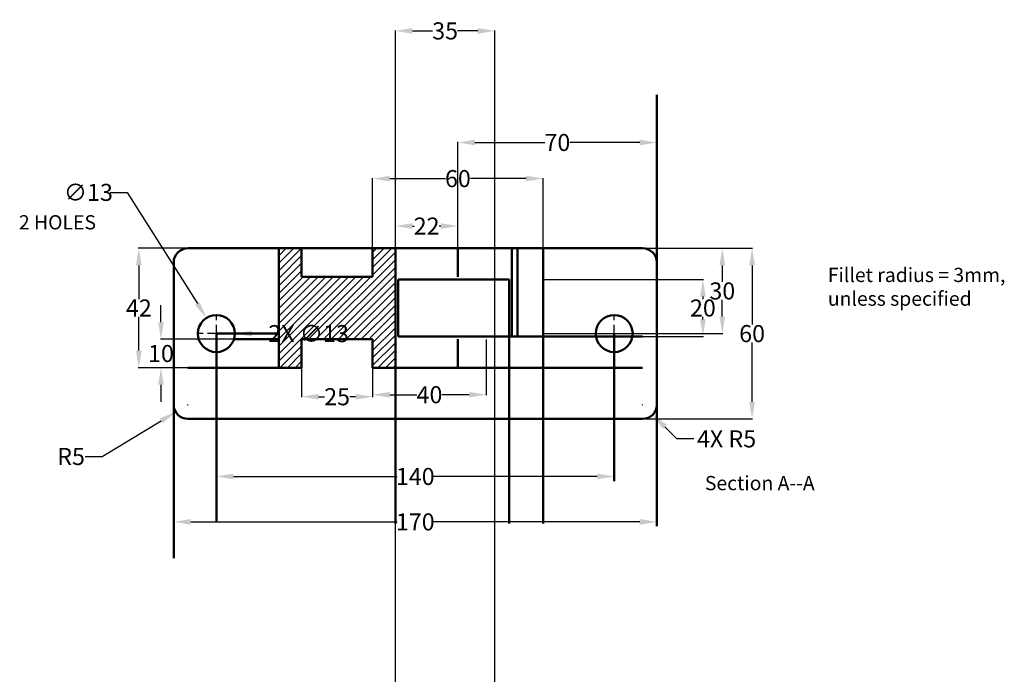
# Model space of a CAD drawing. Units: inches. Extents: x 537 to 975, y 162 to 623.
# Tile 2 of 2: x 537 to 883, y 393 to 623. Entities that reach past the tile are written whole.
import ezdxf

# ---------------------------------------------------------------- set-up
doc = ezdxf.new("R2010")
doc.units = ezdxf.units.IN
doc.header["$LTSCALE"] = 5
doc.header["$MEASUREMENT"] = 0
doc.linetypes.add('HIDDEN2', pattern=[0.1875, 0.125, -0.0625])
for name, color, linetype, lineweight in [('M-DIMS', 2, 'Continuous', 25), ('M-HATC', 8, 'Continuous', 18), ('M-HIDN', 4, 'HIDDEN2', 25), ('M-OUTL', 7, 'Continuous', 50), ('M-TEXT', 3, 'Continuous', 25)]:
    doc.layers.add(name, color=color, linetype=linetype, lineweight=lineweight)
doc.styles.get("Standard").update_dxf_attribs({"font": 'arial.ttf'})
doc.dimstyles.get("Standard").update_dxf_attribs({"dimtxt": 6, "dimasz": 6, "dimexe": 0.18, "dimexo": 0.0625, "dimgap": 0.09, "dimtad": 0, "dimtih": 1, "dimtoh": 1, "dimdec": 0, "dimzin": 0, "dimdsep": 46, "dimtxsty": 'Standard', "dimcen": 0.09, "dimadec": 0, "dimazin": 0, "dimtfac": 1, "dimtdec": 0, "dimtofl": 0, "dimtmove": 0, "dimatfit": 3, "dimfxl": 1, "dimtolj": 1, "dimtzin": 0, "dimarcsym": 0})

# ---------------------------------------------------------------- blocks, each defined once
blk = doc.blocks.new('*D1')
at = {"layer": 'Defpoints', "color": 0, "lineweight": 30, "transparency": 16777216}
for p in [(605.92, 483.04), (745.92, 483.83), (745.92, 462.8)]:
    blk.add_point(p, dxfattribs=at)
at = {"layer": 'M-DIMS', "color": 0, "lineweight": -2, "transparency": 16777216}
for p, q in [((605.92, 482.98), (605.92, 462.62)), ((745.92, 483.77), (745.92, 462.62)), ((611.92, 462.8), (669.49, 462.8)), ((739.92, 462.8), (682.34, 462.8))]:
    blk.add_line(p, q, dxfattribs=at)
at = {"layer": 'M-DIMS', "color": 0, "lineweight": 30, "transparency": 16777216}
for points in [[(611.92, 463.8), (611.92, 461.8), (605.92, 462.8)], [(739.92, 463.8), (739.92, 461.8), (745.92, 462.8)]]:
    blk.add_solid(points, dxfattribs=at)
at = {"layer": 'M-DIMS', "color": 0, "transparency": 16777216, "insert": (675.92, 462.8), "char_height": 6, "attachment_point": 5}
blk.add_mtext('\\A1;140', dxfattribs=at)
blk = doc.blocks.new('*D2')
at = {"layer": 'Defpoints', "color": 0, "lineweight": 30, "transparency": 16777216}
for p in [(760.92, 451.49), (590.92, 448.29), (760.92, 446.82)]:
    blk.add_point(p, dxfattribs=at)
at = {"layer": 'M-DIMS', "color": 0, "lineweight": -2, "transparency": 16777216}
for p, q in [((760.92, 451.43), (760.92, 446.64)), ((590.92, 448.23), (590.92, 446.64)), ((596.92, 446.82), (669.49, 446.82)), ((754.92, 446.82), (682.34, 446.82))]:
    blk.add_line(p, q, dxfattribs=at)
at = {"layer": 'M-DIMS', "color": 0, "lineweight": 30, "transparency": 16777216}
for points in [[(596.92, 447.82), (596.92, 445.82), (590.92, 446.82)], [(754.92, 447.82), (754.92, 445.82), (760.92, 446.82)]]:
    blk.add_solid(points, dxfattribs=at)
at = {"layer": 'M-DIMS', "color": 0, "transparency": 16777216, "insert": (675.92, 446.82), "char_height": 6, "attachment_point": 5}
blk.add_mtext('\\A1;170', dxfattribs=at)
blk = doc.blocks.new('*D3')
at = {"layer": 'Defpoints', "color": 0, "lineweight": 30, "transparency": 16777216}
for p in [(660.92, 511.04), (700.92, 511.04), (700.92, 491.55)]:
    blk.add_point(p, dxfattribs=at)
at = {"layer": 'M-DIMS', "color": 0, "lineweight": -2, "transparency": 16777216}
for p, q in [((660.92, 510.98), (660.92, 491.37)), ((700.92, 510.98), (700.92, 491.37)), ((666.92, 491.55), (676.42, 491.55)), ((694.92, 491.55), (685.41, 491.55))]:
    blk.add_line(p, q, dxfattribs=at)
at = {"layer": 'M-DIMS', "color": 0, "lineweight": 30, "transparency": 16777216}
for points in [[(666.92, 492.55), (666.92, 490.55), (660.92, 491.55)], [(694.92, 492.55), (694.92, 490.55), (700.92, 491.55)]]:
    blk.add_solid(points, dxfattribs=at)
at = {"layer": 'M-DIMS', "color": 0, "transparency": 16777216, "insert": (680.92, 491.55), "char_height": 6, "attachment_point": 5}
blk.add_mtext('\\A1;40', dxfattribs=at)
blk = doc.blocks.new('*D4')
at = {"layer": 'Defpoints', "color": 0, "lineweight": 30, "transparency": 16777216}
for p in [(635.92, 511.04), (660.92, 511.04), (660.92, 490.84)]:
    blk.add_point(p, dxfattribs=at)
at = {"layer": 'M-DIMS', "color": 0, "lineweight": -2, "transparency": 16777216}
for p, q in [((635.92, 510.98), (635.92, 490.66)), ((660.92, 510.98), (660.92, 490.66)), ((641.92, 490.84), (643.95, 490.84)), ((654.92, 490.84), (652.88, 490.84))]:
    blk.add_line(p, q, dxfattribs=at)
at = {"layer": 'M-DIMS', "color": 0, "lineweight": 30, "transparency": 16777216}
for points in [[(641.92, 491.84), (641.92, 489.84), (635.92, 490.84)], [(654.92, 491.84), (654.92, 489.84), (660.92, 490.84)]]:
    blk.add_solid(points, dxfattribs=at)
at = {"layer": 'M-DIMS', "color": 0, "transparency": 16777216, "insert": (648.42, 490.84), "char_height": 6, "attachment_point": 5}
blk.add_mtext('\\A1;25', dxfattribs=at)
blk = doc.blocks.new('*D5')
at = {"layer": 'Defpoints', "color": 0, "lineweight": 30, "transparency": 16777216}
for p in [(690.92, 550.86), (668.92, 543.04), (690.92, 543.04)]:
    blk.add_point(p, dxfattribs=at)
at = {"layer": 'M-DIMS', "color": 0, "lineweight": -2, "transparency": 16777216}
for p, q in [((668.92, 543.11), (668.92, 551.04)), ((674.92, 550.86), (675.51, 550.86)), ((684.92, 550.86), (684.32, 550.86)), ((690.92, 543.11), (690.92, 551.04))]:
    blk.add_line(p, q, dxfattribs=at)
at = {"layer": 'M-DIMS', "color": 0, "lineweight": 30, "transparency": 16777216}
for points in [[(674.92, 551.86), (674.92, 549.86), (668.92, 550.86)], [(684.92, 551.86), (684.92, 549.86), (690.92, 550.86)]]:
    blk.add_solid(points, dxfattribs=at)
at = {"layer": 'M-DIMS', "color": 0, "transparency": 16777216, "insert": (679.92, 550.86), "char_height": 6, "attachment_point": 5}
blk.add_mtext('\\A1;22', dxfattribs=at)
blk = doc.blocks.new('*D6')
at = {"layer": 'Defpoints', "color": 0, "lineweight": 30, "transparency": 16777216}
for p in [(720.92, 567.55), (660.92, 543.04), (720.92, 543.04)]:
    blk.add_point(p, dxfattribs=at)
at = {"layer": 'M-DIMS', "color": 0, "lineweight": -2, "transparency": 16777216}
for p, q in [((660.92, 543.11), (660.92, 567.73)), ((666.92, 567.55), (686.52, 567.55)), ((714.92, 567.55), (695.31, 567.55)), ((720.92, 543.11), (720.92, 567.73))]:
    blk.add_line(p, q, dxfattribs=at)
at = {"layer": 'M-DIMS', "color": 0, "lineweight": 30, "transparency": 16777216}
for points in [[(666.92, 568.55), (666.92, 566.55), (660.92, 567.55)], [(714.92, 568.55), (714.92, 566.55), (720.92, 567.55)]]:
    blk.add_solid(points, dxfattribs=at)
at = {"layer": 'M-DIMS', "color": 0, "transparency": 16777216, "insert": (690.92, 567.55), "char_height": 6, "attachment_point": 5}
blk.add_mtext('\\A1;60', dxfattribs=at)
blk = doc.blocks.new('*D7')
at = {"layer": 'Defpoints', "color": 0, "lineweight": 30, "transparency": 16777216}
for p in [(760.92, 580.25), (690.92, 551.04), (760.92, 551.04)]:
    blk.add_point(p, dxfattribs=at)
at = {"layer": 'M-DIMS', "color": 0, "lineweight": -2, "transparency": 16777216}
for p, q in [((690.92, 551.1), (690.92, 580.43)), ((696.92, 580.25), (721.56, 580.25)), ((754.92, 580.25), (730.27, 580.25)), ((760.92, 551.1), (760.92, 580.43))]:
    blk.add_line(p, q, dxfattribs=at)
at = {"layer": 'M-DIMS', "color": 0, "lineweight": 30, "transparency": 16777216}
for points in [[(696.92, 581.25), (696.92, 579.25), (690.92, 580.25)], [(754.92, 581.25), (754.92, 579.25), (760.92, 580.25)]]:
    blk.add_solid(points, dxfattribs=at)
at = {"layer": 'M-DIMS', "color": 0, "transparency": 16777216, "insert": (725.92, 580.25), "char_height": 6, "attachment_point": 5}
blk.add_mtext('\\A1;70', dxfattribs=at)
blk = doc.blocks.new('*D8')
at = {"layer": 'Defpoints', "color": 0, "lineweight": 30, "transparency": 16777216}
for p in [(578.65, 543.04), (605.92, 543.04), (605.92, 501.04)]:
    blk.add_point(p, dxfattribs=at)
at = {"layer": 'M-DIMS', "color": 0, "lineweight": -2, "transparency": 16777216}
for p, q in [((605.85, 543.04), (578.47, 543.04)), ((578.65, 537.04), (578.65, 525.14)), ((578.65, 507.04), (578.65, 518.94)), ((605.85, 501.04), (578.47, 501.04))]:
    blk.add_line(p, q, dxfattribs=at)
at = {"layer": 'M-DIMS', "color": 0, "lineweight": 30, "transparency": 16777216}
for points in [[(577.65, 537.04), (579.65, 537.04), (578.65, 543.04)], [(577.65, 507.04), (579.65, 507.04), (578.65, 501.04)]]:
    blk.add_solid(points, dxfattribs=at)
at = {"layer": 'M-DIMS', "color": 0, "transparency": 16777216, "insert": (578.65, 522.04), "char_height": 6, "attachment_point": 5}
blk.add_mtext('\\A1;42', dxfattribs=at)
blk = doc.blocks.new('*D9')
at = {"layer": 'Defpoints', "color": 0, "lineweight": 30, "transparency": 16777216}
for p in [(586.44, 511.04), (627.92, 511.04), (627.92, 501.04)]:
    blk.add_point(p, dxfattribs=at)
at = {"layer": 'M-DIMS', "color": 0, "lineweight": -2, "transparency": 16777216}
for p, q in [((586.44, 517.04), (586.44, 523.04)), ((627.85, 511.04), (586.26, 511.04)), ((627.85, 501.04), (586.26, 501.04)), ((586.44, 495.04), (586.44, 489.04))]:
    blk.add_line(p, q, dxfattribs=at)
at = {"layer": 'M-DIMS', "color": 0, "lineweight": 30, "transparency": 16777216}
for points in [[(585.44, 517.04), (587.44, 517.04), (586.44, 511.04)], [(585.44, 495.04), (587.44, 495.04), (586.44, 501.04)]]:
    blk.add_solid(points, dxfattribs=at)
at = {"layer": 'M-DIMS', "color": 0, "transparency": 16777216, "insert": (586.44, 506.04), "char_height": 6, "attachment_point": 5}
blk.add_mtext('\\A1;10', dxfattribs=at)
blk = doc.blocks.new('*D10')
at = {"layer": 'Defpoints', "color": 0, "lineweight": 30, "transparency": 16777216}
for p in [(720.92, 543.04), (720.92, 513.04), (783.95, 513.04)]:
    blk.add_point(p, dxfattribs=at)
at = {"layer": 'M-DIMS', "color": 0, "lineweight": -2, "transparency": 16777216}
for p, q in [((720.98, 543.04), (784.13, 543.04)), ((783.95, 537.04), (783.95, 531.2)), ((783.95, 519.04), (783.95, 524.89)), ((720.98, 513.04), (784.13, 513.04))]:
    blk.add_line(p, q, dxfattribs=at)
at = {"layer": 'M-DIMS', "color": 0, "lineweight": 30, "transparency": 16777216}
for points in [[(782.95, 537.04), (784.95, 537.04), (783.95, 543.04)], [(782.95, 519.04), (784.95, 519.04), (783.95, 513.04)]]:
    blk.add_solid(points, dxfattribs=at)
at = {"layer": 'M-DIMS', "color": 0, "transparency": 16777216, "insert": (783.95, 528.04), "char_height": 6, "attachment_point": 5}
blk.add_mtext('\\A1;30', dxfattribs=at)
blk = doc.blocks.new('*D11')
at = {"layer": 'Defpoints', "color": 0, "lineweight": 30, "transparency": 16777216}
for p in [(720.92, 532.04), (777.12, 532.04), (720.92, 512.04)]:
    blk.add_point(p, dxfattribs=at)
at = {"layer": 'M-DIMS', "color": 0, "lineweight": -2, "transparency": 16777216}
for p, q in [((720.98, 532.04), (777.3, 532.04)), ((777.12, 526.04), (777.12, 525.2)), ((777.12, 518.04), (777.12, 518.89)), ((720.98, 512.04), (777.3, 512.04))]:
    blk.add_line(p, q, dxfattribs=at)
at = {"layer": 'M-DIMS', "color": 0, "lineweight": 30, "transparency": 16777216}
for points in [[(776.12, 526.04), (778.12, 526.04), (777.12, 532.04)], [(776.12, 518.04), (778.12, 518.04), (777.12, 512.04)]]:
    blk.add_solid(points, dxfattribs=at)
at = {"layer": 'M-DIMS', "color": 0, "transparency": 16777216, "insert": (777.12, 522.04), "char_height": 6, "attachment_point": 5}
blk.add_mtext('\\A1;20', dxfattribs=at)
blk = doc.blocks.new('*D12')
at = {"layer": 'Defpoints', "color": 0, "lineweight": 30, "transparency": 16777216}
for p in [(722.98, 543.04), (794.43, 543.04), (722.98, 483.04)]:
    blk.add_point(p, dxfattribs=at)
at = {"layer": 'M-DIMS', "color": 0, "lineweight": -2, "transparency": 16777216}
for p, q in [((723.04, 543.04), (794.61, 543.04)), ((794.43, 537.04), (794.43, 516.2)), ((794.43, 489.04), (794.43, 509.89)), ((723.04, 483.04), (794.61, 483.04))]:
    blk.add_line(p, q, dxfattribs=at)
at = {"layer": 'M-DIMS', "color": 0, "lineweight": 30, "transparency": 16777216}
for points in [[(793.43, 537.04), (795.43, 537.04), (794.43, 543.04)], [(793.43, 489.04), (795.43, 489.04), (794.43, 483.04)]]:
    blk.add_solid(points, dxfattribs=at)
at = {"layer": 'M-DIMS', "color": 0, "transparency": 16777216, "insert": (794.43, 513.04), "char_height": 6, "attachment_point": 5}
blk.add_mtext('\\A1;60', dxfattribs=at)
blk = doc.blocks.new('*D13')
at = {"layer": 'Defpoints', "color": 0, "lineweight": 30, "ltscale": 5, "transparency": 16777216}
for p in [(602.45, 518.54), (609.39, 507.55)]:
    blk.add_point(p, dxfattribs=at)
at = {"layer": 'M-DIMS', "color": 0, "lineweight": -2, "ltscale": 5, "transparency": 16777216}
for p, q in [((568.55, 562.71), (574.55, 562.71)), ((574.55, 562.71), (599.24, 523.61)), ((605.83, 513.04), (606.01, 513.04)), ((605.92, 512.95), (605.92, 513.13))]:
    blk.add_line(p, q, dxfattribs=at)
at = {"layer": 'M-DIMS', "color": 0, "lineweight": 30, "ltscale": 5, "transparency": 16777216}
blk.add_solid([(600.09, 524.15), (598.4, 523.08), (602.45, 518.54)], dxfattribs=at)
at = {"layer": 'M-DIMS', "color": 0, "ltscale": 5, "transparency": 16777216, "insert": (560.89, 562.71), "char_height": 6, "attachment_point": 5}
blk.add_mtext('\\A1;∅13', dxfattribs=at)
blk = doc.blocks.new('*D14')
at = {"layer": 'Defpoints', "color": 0, "lineweight": 30, "ltscale": 5, "transparency": 16777216}
for p in [(591.64, 485.46), (595.92, 488.04)]:
    blk.add_point(p, dxfattribs=at)
at = {"layer": 'M-DIMS', "color": 0, "lineweight": -2, "ltscale": 5, "transparency": 16777216}
for p, q in [((595.83, 488.04), (596.01, 488.04)), ((595.92, 487.95), (595.92, 488.13)), ((565.76, 469.82), (586.5, 482.35)), ((559.76, 469.82), (565.76, 469.82))]:
    blk.add_line(p, q, dxfattribs=at)
at = {"layer": 'M-DIMS', "color": 0, "lineweight": 30, "ltscale": 5, "transparency": 16777216}
blk.add_solid([(585.98, 483.21), (587.02, 481.5), (591.64, 485.46)], dxfattribs=at)
at = {"layer": 'M-DIMS', "color": 0, "ltscale": 5, "transparency": 16777216, "insert": (554.81, 469.82), "char_height": 6, "attachment_point": 5}
blk.add_mtext('\\A1;R5', dxfattribs=at)
blk = doc.blocks.new('*D33')
at = {"layer": 'Defpoints', "color": 0, "lineweight": 30, "ltscale": 5, "transparency": 16777216}
for p in [(703.92, 619.5), (668.92, 365.97), (703.92, 365.97)]:
    blk.add_point(p, dxfattribs=at)
at = {"layer": 'M-DIMS', "color": 0, "lineweight": -2, "ltscale": 5, "transparency": 16777216}
for p, q in [((668.92, 366.03), (668.92, 619.68)), ((674.92, 619.5), (682.01, 619.5)), ((697.92, 619.5), (690.82, 619.5)), ((703.92, 366.03), (703.92, 619.68))]:
    blk.add_line(p, q, dxfattribs=at)
at = {"layer": 'M-DIMS', "color": 0, "lineweight": 30, "ltscale": 5, "transparency": 16777216}
for points in [[(674.92, 620.5), (674.92, 618.5), (668.92, 619.5)], [(697.92, 620.5), (697.92, 618.5), (703.92, 619.5)]]:
    blk.add_solid(points, dxfattribs=at)
at = {"layer": 'M-DIMS', "color": 0, "ltscale": 5, "transparency": 16777216, "insert": (686.42, 619.5), "char_height": 6, "attachment_point": 5}
blk.add_mtext('\\A1;35', dxfattribs=at)
blk = doc.blocks.new('*D39')
at = {"layer": 'Defpoints', "color": 0, "lineweight": 30, "ltscale": 5, "transparency": 16777216}
for p in [(599.42, 513.04), (612.42, 513.04)]:
    blk.add_point(p, dxfattribs=at)
at = {"layer": 'M-DIMS', "color": 0, "lineweight": -2, "ltscale": 5, "transparency": 16777216}
for p, q in [((605.83, 513.04), (606.01, 513.04)), ((605.92, 512.95), (605.92, 513.13)), ((624.42, 513.04), (618.42, 513.04))]:
    blk.add_line(p, q, dxfattribs=at)
at = {"layer": 'M-DIMS', "color": 0, "lineweight": 30, "ltscale": 5, "transparency": 16777216}
blk.add_solid([(618.42, 514.04), (618.42, 512.04), (612.42, 513.04)], dxfattribs=at)
at = {"layer": 'M-DIMS', "color": 0, "ltscale": 5, "transparency": 16777216, "insert": (638.4, 513.04), "char_height": 6, "attachment_point": 5}
blk.add_mtext('\\A1;2X ∅13', dxfattribs=at)
blk = doc.blocks.new('*D40')
at = {"layer": 'Defpoints', "color": 0, "lineweight": 30, "ltscale": 5, "transparency": 16777216}
for p in [(755.92, 488.04), (759.45, 484.51)]:
    blk.add_point(p, dxfattribs=at)
at = {"layer": 'M-DIMS', "color": 0, "lineweight": -2, "ltscale": 5, "transparency": 16777216}
for p, q in [((755.83, 488.04), (756.01, 488.04)), ((755.92, 487.95), (755.92, 488.13)), ((767.94, 476.02), (763.69, 480.26)), ((773.94, 476.02), (767.94, 476.02))]:
    blk.add_line(p, q, dxfattribs=at)
at = {"layer": 'M-DIMS', "color": 0, "lineweight": 30, "ltscale": 5, "transparency": 16777216}
blk.add_solid([(764.4, 480.97), (762.99, 479.56), (759.45, 484.51)], dxfattribs=at)
at = {"layer": 'M-DIMS', "color": 0, "ltscale": 5, "transparency": 16777216, "insert": (785.45, 476.02), "char_height": 6, "attachment_point": 5}
blk.add_mtext('\\A1;4X R5', dxfattribs=at)

msp = doc.modelspace()

# ---------------------------------------------------------------- hatches: boundary and pattern name
at = {"layer": 'M-HATC', "ltscale": 5}
h = msp.add_hatch(dxfattribs=at)
h.set_pattern_fill('ANSI31', color=256, scale=15)
h.paths.add_polyline_path([(668.92, 543.04), (660.92, 543.04), (660.92, 533.04), (635.92, 533.04), (635.92, 543.04), (627.92, 543.04), (627.92, 501.04), (635.92, 501.04), (635.92, 511.04), (660.92, 511.04), (660.92, 501.04), (668.92, 501.04)])

# ---------------------------------------------------------------- linework, layer by layer
at = {"layer": 'M-HIDN', "ltscale": 5}
for p, q in [((605.92, 513.04), (605.92, 519.54)), ((745.92, 513.04), (745.92, 519.54)), ((605.92, 513.04), (599.42, 513.04)), ((745.92, 513.04), (752.56, 513.04))]:
    msp.add_line(p, q, dxfattribs=at)
at = {"layer": 'M-OUTL'}
for p, q in [((760.92, 513.04), (760.92, 597)), ((660.92, 543.04), (595.92, 543.04)), ((627.92, 501.04), (627.92, 543.04)), ((635.92, 533.04), (635.92, 543.04)), ((755.92, 543.04), (660.92, 543.04)), ((660.92, 533.04), (660.92, 543.04)), ((668.92, 501.04), (668.92, 543.04)), ((690.92, 533.04), (690.92, 543.04)), ((709.92, 512.04), (709.92, 543.04)), ((711.92, 512.04), (711.92, 543.04)), ((720.92, 512.04), (720.92, 543.04)), ((590.92, 538.04), (590.92, 488.04)), ((760.92, 488.04), (760.92, 538.04)), ((660.92, 533.04), (635.92, 533.04)), ((660.92, 533.04), (635.92, 533.04)), ((669.92, 512.04), (669.92, 532.04)), ((690.92, 532.04), (669.92, 532.04)), ((690.92, 532.04), (708.92, 532.04)), ((708.92, 512.04), (708.92, 532.04)), ((605.92, 513.04), (605.92, 506.54)), ((605.92, 513.04), (612.42, 513.04)), ((627.92, 513.04), (612.42, 513.04)), ((745.92, 513.04), (745.92, 506.54)), ((627.92, 511.04), (612.1, 511.04)), ((635.92, 501.04), (635.92, 511.04)), ((660.92, 511.04), (635.92, 511.04)), ((660.92, 501.04), (660.92, 511.04)), ((690.92, 512.04), (669.92, 512.04)), ((690.92, 512.04), (711.92, 512.04)), ((690.92, 511.04), (690.92, 501.04)), ((755.92, 512.04), (708.92, 512.04)), ((605.92, 506.54), (605.92, 446.68)), ((745.92, 506.54), (745.92, 461.12)), ((635.92, 501.04), (595.92, 501.04)), ((755.92, 501.04), (660.92, 501.04)), ((590.92, 488.04), (590.92, 434.03)), ((760.92, 488.04), (760.92, 445.35)), ((595.92, 483.04), (755.92, 483.04))]:
    msp.add_line(p, q, dxfattribs=at)
at = {"layer": 'M-OUTL', "ltscale": 5}
for p, q in [((708.92, 512.04), (708.92, 446.31)), ((720.92, 512.04), (720.92, 446.31)), ((668.92, 501.04), (668.92, 446.31))]:
    msp.add_line(p, q, dxfattribs=at)
at = {"layer": 'M-OUTL'}
for centre in [(605.92, 513.04), (745.92, 513.04)]:
    msp.add_circle(centre, 6.5, dxfattribs=at)
for centre, start, end in [((595.92, 538.04), 90, 180), ((755.92, 538.04), 0, 90), ((595.92, 488.04), 180, 270), ((755.92, 488.04), 270, 0)]:
    msp.add_arc(centre, 5, start, end, dxfattribs=at)

# ---------------------------------------------------------------- texts
at = {"layer": 'M-TEXT', "ltscale": 5, "char_height": 5, "attachment_point": 1}
for s, width, insert in [('2 HOLES', 46.6378, (536.45, 554.69)), ('Fillet radius = 3mm,\\Punless specified', 94.2525, (821.09, 536.17)), ('Section A--A', 46.6378, (777.82, 462.96))]:
    msp.add_mtext_dynamic_manual_height_columns(s, width=width, gutter_width=1, heights=[0], dxfattribs=dict(at, insert=insert))

# ---------------------------------------------------------------- dimensions: what is measured, and where the dimension line sits
at = {"layer": 'M-DIMS', "ltscale": 5}
dim = msp.add_linear_dim(base=(703.92, 619.5), p1=(668.92, 365.97), p2=(703.92, 365.97), dimstyle='Standard', override={"dimdec": 0, "dimlfac": 1, "dimrnd": 0, "dimzin": 0, "dimdsep": 46, "dimlunit": 2}, dxfattribs=at)
dim.commit()
dim.dimension.update_dxf_attribs({"geometry": '*D33', "text_midpoint": (686.42, 619.5)})
at = {"layer": 'M-DIMS'}
for base, p1, p2, picture, middle in [((760.92, 580.25), (690.92, 551.04), (760.92, 551.04), '*D7', (725.92, 580.25)), ((720.92, 567.55), (660.92, 543.04), (720.92, 543.04), '*D6', (690.92, 567.55)), ((690.92, 550.86), (668.92, 543.04), (690.92, 543.04), '*D5', (679.92, 550.86)), ((660.92, 490.84), (635.92, 511.04), (660.92, 511.04), '*D4', (648.42, 490.84)), ((700.92, 491.55), (660.92, 511.04), (700.92, 511.04), '*D3', (680.92, 491.55)), ((745.92, 462.8), (605.92, 483.04), (745.92, 483.83), '*D1', (675.92, 462.8)), ((760.92, 446.82), (590.92, 448.29), (760.92, 451.49), '*D2', (675.92, 446.82))]:
    dim = msp.add_linear_dim(base=base, p1=p1, p2=p2, dimstyle='Standard', override={"dimclrd": 0, "dimclre": 0, "dimclrt": 0}, dxfattribs=at)
    dim.commit()
    dim.dimension.update_dxf_attribs({"geometry": picture, "text_midpoint": middle})
at = {"layer": 'M-DIMS', "ltscale": 5}
dim = msp.add_diameter_dim_2p(p1=(609.39, 507.55), p2=(602.45, 518.54), dimstyle='Standard', override={"dimclrd": 0, "dimclre": 0, "dimclrt": 0}, dxfattribs=at)
dim.commit()
dim.dimension.update_dxf_attribs({"geometry": '*D13', "text_midpoint": (560.89, 562.71), "dimtype": 163})
at = {"layer": 'M-DIMS'}
for base, p1, p2, picture, middle in [((578.65, 543.04), (605.92, 501.04), (605.92, 543.04), '*D8', (578.65, 522.04)), ((783.95, 513.04), (720.92, 543.04), (720.92, 513.04), '*D10', (783.95, 528.04)), ((794.43, 543.04), (722.98, 483.04), (722.98, 543.04), '*D12', (794.43, 513.04)), ((777.12, 532.04), (720.92, 512.04), (720.92, 532.04), '*D11', (777.12, 522.04)), ((586.44, 511.04), (627.92, 501.04), (627.92, 511.04), '*D9', (586.44, 506.04))]:
    dim = msp.add_linear_dim(base=base, p1=p1, p2=p2, angle=90, dimstyle='Standard', override={"dimclrd": 0, "dimclre": 0, "dimclrt": 0}, dxfattribs=at)
    dim.commit()
    dim.dimension.update_dxf_attribs({"geometry": picture, "text_midpoint": middle})
at = {"layer": 'M-DIMS', "ltscale": 5}
dim = msp.add_diameter_dim_2p(p1=(599.42, 513.04), p2=(612.42, 513.04), text='2X <>', dimstyle='Standard', override={"dimdec": 0, "dimlfac": 1, "dimrnd": 0, "dimzin": 0, "dimdsep": 46, "dimlunit": 2}, dxfattribs=at)
dim.commit()
dim.dimension.update_dxf_attribs({"geometry": '*D39', "text_midpoint": (624.42, 513.04), "dimtype": 163})
dim = msp.add_radius_dim(center=(595.92, 488.04), mpoint=(591.64, 485.46), dimstyle='Standard', override={"dimclrd": 0, "dimclre": 0, "dimclrt": 0}, dxfattribs=at)
dim.commit()
dim.dimension.update_dxf_attribs({"geometry": '*D14', "text_midpoint": (554.81, 469.82), "dimtype": 164})
dim = msp.add_radius_dim(center=(755.92, 488.04), mpoint=(759.45, 484.51), text='4X <>', dimstyle='Standard', override={"dimdec": 0, "dimlfac": 1, "dimrnd": 0, "dimzin": 0, "dimdsep": 46, "dimlunit": 2}, dxfattribs=at)
dim.commit()
dim.dimension.update_dxf_attribs({"geometry": '*D40', "text_midpoint": (785.45, 476.02)})

doc.saveas('drawing.dxf')
